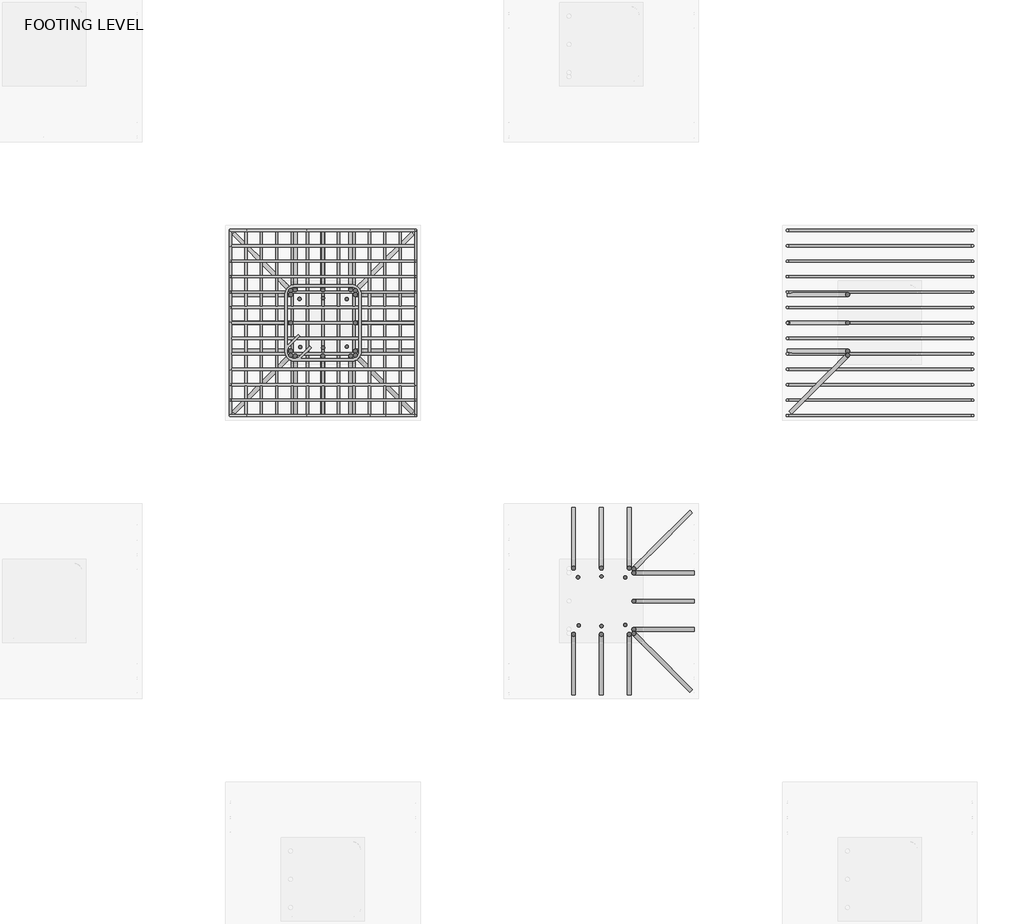
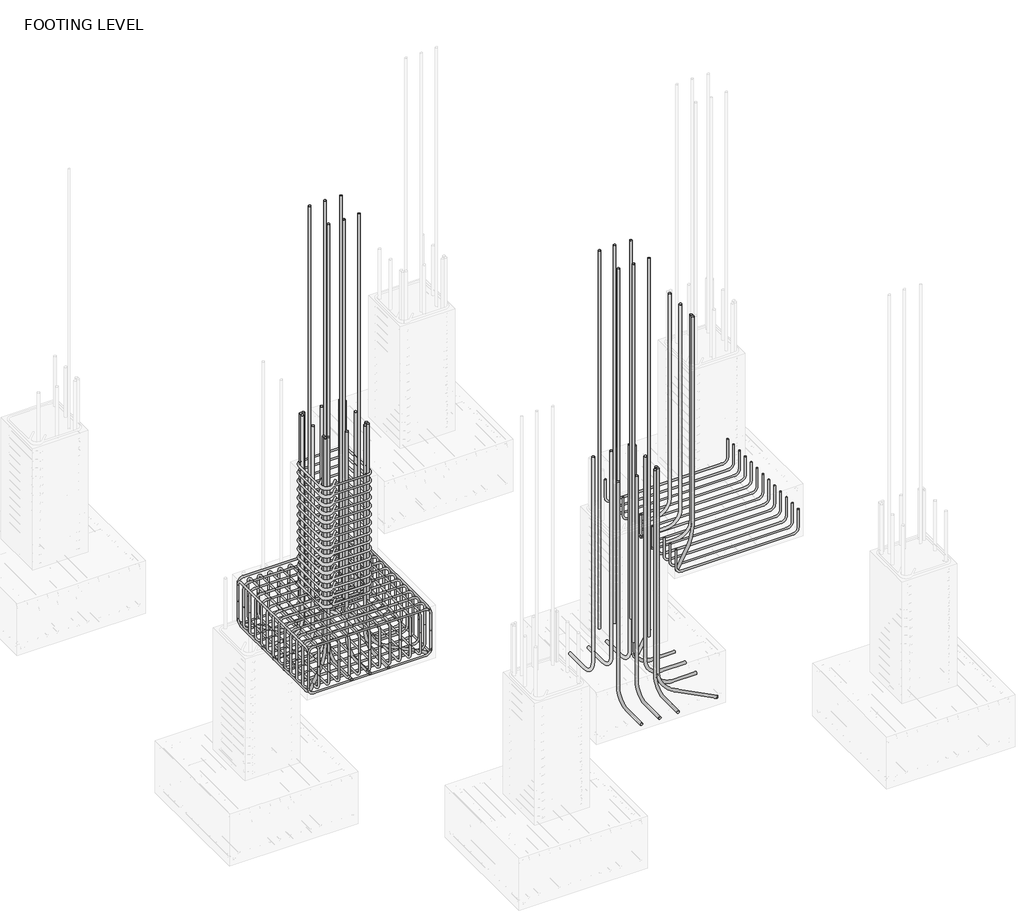
# One storey, part 6 of 10: 34 reinforcing bars.
"""IFC4 building model written with IfcOpenShell, lengths in millimetres."""

from ifc_helpers import new_model, si_unit, point, frame, origin, place, context, project, spatial, polyline, circle_curve, trimmed, segment, composite_curve, source, transform, mapped, element, save
from ifc_brep_helpers import swept_disk

model = new_model("IFC4")

# Units and contexts
model_context = context("Model", 3, world=origin())
ifc_project = project(units=[si_unit("LENGTHUNIT", "METRE", prefix="MILLI")], contexts=[model_context])

# Site, building, storey
site = spatial("IfcSite", under=ifc_project)
building = spatial("IfcBuilding", under=site)
storey = spatial("IfcBuildingStorey", under=building, Name="FOOTING LEVEL", Elevation=-2133.6)

# Reinforcing bars
placement = place(None, origin())
reinforcing_bar_shape = source(origin(), model_context, "Body", "SolidModel", [
    swept_disk(composite_curve([segment(polyline([(365.0730963, 6852.4829396, -2583.0), (365.0730963, 6852.4829396, -2905.1)]), True, "CONTINUOUS"), segment(trimmed(circle_curve(frame((274.8730963, 6852.4829396, -2905.1), z_axis=(0.0, 1.0, 0.0), x_axis=(90.19999999999999, 0.0, 0.0)), 90.2), [point((365.0730963, 6852.4829396, -2905.1))], [point((274.8730963, 6852.4829396, -2995.3))], True, "CARTESIAN"), True, "CONTINUOUS"), segment(polyline([(274.8730963, 6852.4829396, -2995.3), (-1572.9269037, 6852.4829396, -2995.3)]), True, "CONTINUOUS"), segment(trimmed(circle_curve(frame((-1572.9269037, 6852.4829396, -2905.1), z_axis=(0.0, 1.0, 0.0), x_axis=(0.0, 0.0, -90.20000000000027)), 90.2), [point((-1572.9269037, 6852.4829396, -2995.3))], [point((-1663.1269037, 6852.4829396, -2905.1))], True, "CARTESIAN"), True, "CONTINUOUS"), segment(polyline([(-1663.1269037, 6852.4829396, -2905.1), (-1663.1269037, 6852.4829396, -2583.0)]), True, "CONTINUOUS")], self_intersect=False), 12.7),
])
element("IfcReinforcingBar", 1, at=placement, inside=storey, context=model_context, shape_type="MappedRepresentation", body=[
    mapped(reinforcing_bar_shape, transform((0.0, 0.0, 0.0), x_axis=(1.0, 0.0, 0.0), y_axis=(0.0, 1.0, 0.0), z_axis=(0.0, 0.0, 1.0))),
    mapped(reinforcing_bar_shape, transform((0.0, -169.0166667, 0.0), x_axis=(1.0, 0.0, 0.0), y_axis=(0.0, 1.0, 0.0), z_axis=(0.0, 0.0, 1.0))),
    mapped(reinforcing_bar_shape, transform((0.0, -338.0333333, 0.0), x_axis=(1.0, 0.0, 0.0), y_axis=(0.0, 1.0, 0.0), z_axis=(0.0, 0.0, 1.0))),
    mapped(reinforcing_bar_shape, transform((0.0, -507.05, 0.0), x_axis=(1.0, 0.0, 0.0), y_axis=(0.0, 1.0, 0.0), z_axis=(0.0, 0.0, 1.0))),
    mapped(reinforcing_bar_shape, transform((0.0, -676.0666667, 0.0), x_axis=(1.0, 0.0, 0.0), y_axis=(0.0, 1.0, 0.0), z_axis=(0.0, 0.0, 1.0))),
    mapped(reinforcing_bar_shape, transform((0.0, -845.0833333, 0.0), x_axis=(1.0, 0.0, 0.0), y_axis=(0.0, 1.0, 0.0), z_axis=(0.0, 0.0, 1.0))),
    mapped(reinforcing_bar_shape, transform((0.0, -1014.1, 0.0), x_axis=(1.0, 0.0, 0.0), y_axis=(0.0, 1.0, 0.0), z_axis=(0.0, 0.0, 1.0))),
    mapped(reinforcing_bar_shape, transform((0.0, -1183.1166667, 0.0), x_axis=(1.0, 0.0, 0.0), y_axis=(0.0, 1.0, 0.0), z_axis=(0.0, 0.0, 1.0))),
    mapped(reinforcing_bar_shape, transform((0.0, -1352.1333333, 0.0), x_axis=(1.0, 0.0, 0.0), y_axis=(0.0, 1.0, 0.0), z_axis=(0.0, 0.0, 1.0))),
    mapped(reinforcing_bar_shape, transform((0.0, -1521.15, 0.0), x_axis=(1.0, 0.0, 0.0), y_axis=(0.0, 1.0, 0.0), z_axis=(0.0, 0.0, 1.0))),
    mapped(reinforcing_bar_shape, transform((0.0, -1690.1666667, 0.0), x_axis=(1.0, 0.0, 0.0), y_axis=(0.0, 1.0, 0.0), z_axis=(0.0, 0.0, 1.0))),
    mapped(reinforcing_bar_shape, transform((0.0, -1859.1833333, 0.0), x_axis=(1.0, 0.0, 0.0), y_axis=(0.0, 1.0, 0.0), z_axis=(0.0, 0.0, 1.0))),
    mapped(reinforcing_bar_shape, transform((0.0, -2028.2, 0.0), x_axis=(1.0, 0.0, 0.0), y_axis=(0.0, 1.0, 0.0), z_axis=(0.0, 0.0, 1.0))),
])
reinforcing_bar_2_shape = source(origin(), model_context, "Body", "SolidModel", [
    swept_disk(composite_curve([segment(polyline([(-5730.9269037, 6852.4829396, -2583.0), (-5730.9269037, 6852.4829396, -2905.1)]), True, "CONTINUOUS"), segment(trimmed(circle_curve(frame((-5821.1269037, 6852.4829396, -2905.1), z_axis=(0.0, 1.0, 0.0), x_axis=(90.19999999999982, 0.0, 0.0)), 90.2), [point((-5730.9269037, 6852.4829396, -2905.1))], [point((-5821.1269037, 6852.4829396, -2995.3))], True, "CARTESIAN"), True, "CONTINUOUS"), segment(polyline([(-5821.1269037, 6852.4829396, -2995.3), (-7668.9269037, 6852.4829396, -2995.3)]), True, "CONTINUOUS"), segment(trimmed(circle_curve(frame((-7668.9269037, 6852.4829396, -2905.1), z_axis=(0.0, 1.0, 0.0), x_axis=(0.0, 0.0, -90.20000000000027)), 90.2), [point((-7668.9269037, 6852.4829396, -2995.3))], [point((-7759.1269037, 6852.4829396, -2905.1))], True, "CARTESIAN"), True, "CONTINUOUS"), segment(polyline([(-7759.1269037, 6852.4829396, -2905.1), (-7759.1269037, 6852.4829396, -2583.0)]), True, "CONTINUOUS")], self_intersect=False), 12.7),
])
element("IfcReinforcingBar", 2, at=placement, inside=storey, context=model_context, shape_type="MappedRepresentation", body=[
    mapped(reinforcing_bar_2_shape, transform((0.0, 0.0, 0.0), x_axis=(1.0, 0.0, 0.0), y_axis=(0.0, 1.0, 0.0), z_axis=(0.0, 0.0, 1.0))),
    mapped(reinforcing_bar_2_shape, transform((0.0, -169.0166667, 0.0), x_axis=(1.0, 0.0, 0.0), y_axis=(0.0, 1.0, 0.0), z_axis=(0.0, 0.0, 1.0))),
    mapped(reinforcing_bar_2_shape, transform((0.0, -338.0333333, 0.0), x_axis=(1.0, 0.0, 0.0), y_axis=(0.0, 1.0, 0.0), z_axis=(0.0, 0.0, 1.0))),
    mapped(reinforcing_bar_2_shape, transform((0.0, -507.05, 0.0), x_axis=(1.0, 0.0, 0.0), y_axis=(0.0, 1.0, 0.0), z_axis=(0.0, 0.0, 1.0))),
    mapped(reinforcing_bar_2_shape, transform((0.0, -676.0666667, 0.0), x_axis=(1.0, 0.0, 0.0), y_axis=(0.0, 1.0, 0.0), z_axis=(0.0, 0.0, 1.0))),
    mapped(reinforcing_bar_2_shape, transform((0.0, -845.0833333, 0.0), x_axis=(1.0, 0.0, 0.0), y_axis=(0.0, 1.0, 0.0), z_axis=(0.0, 0.0, 1.0))),
    mapped(reinforcing_bar_2_shape, transform((0.0, -1014.1, 0.0), x_axis=(1.0, 0.0, 0.0), y_axis=(0.0, 1.0, 0.0), z_axis=(0.0, 0.0, 1.0))),
    mapped(reinforcing_bar_2_shape, transform((0.0, -1183.1166667, 0.0), x_axis=(1.0, 0.0, 0.0), y_axis=(0.0, 1.0, 0.0), z_axis=(0.0, 0.0, 1.0))),
    mapped(reinforcing_bar_2_shape, transform((0.0, -1352.1333333, 0.0), x_axis=(1.0, 0.0, 0.0), y_axis=(0.0, 1.0, 0.0), z_axis=(0.0, 0.0, 1.0))),
    mapped(reinforcing_bar_2_shape, transform((0.0, -1521.15, 0.0), x_axis=(1.0, 0.0, 0.0), y_axis=(0.0, 1.0, 0.0), z_axis=(0.0, 0.0, 1.0))),
    mapped(reinforcing_bar_2_shape, transform((0.0, -1690.1666667, 0.0), x_axis=(1.0, 0.0, 0.0), y_axis=(0.0, 1.0, 0.0), z_axis=(0.0, 0.0, 1.0))),
    mapped(reinforcing_bar_2_shape, transform((0.0, -1859.1833333, 0.0), x_axis=(1.0, 0.0, 0.0), y_axis=(0.0, 1.0, 0.0), z_axis=(0.0, 0.0, 1.0))),
    mapped(reinforcing_bar_2_shape, transform((0.0, -2028.2, 0.0), x_axis=(1.0, 0.0, 0.0), y_axis=(0.0, 1.0, 0.0), z_axis=(0.0, 0.0, 1.0))),
])
reinforcing_bar_3_shape = source(origin(), model_context, "Body", "SolidModel", [
    swept_disk(composite_curve([segment(polyline([(-7759.1269037, 6852.4829396, -2598.6), (-7759.1269037, 6852.4829396, -2276.5)]), True, "CONTINUOUS"), segment(trimmed(circle_curve(frame((-7668.9269037, 6852.4829396, -2276.5), z_axis=(0.0, 1.0, 0.0), x_axis=(-90.19999999999982, 0.0, 0.0)), 90.2), [point((-7759.1269037, 6852.4829396, -2276.5))], [point((-7668.9269037, 6852.4829396, -2186.3))], True, "CARTESIAN"), True, "CONTINUOUS"), segment(polyline([(-7668.9269037, 6852.4829396, -2186.3), (-5821.1269037, 6852.4829396, -2186.3)]), True, "CONTINUOUS"), segment(trimmed(circle_curve(frame((-5821.1269037, 6852.4829396, -2276.5), z_axis=(0.0, 1.0, 0.0), x_axis=(0.0, 0.0, 90.19999999999982)), 90.2), [point((-5821.1269037, 6852.4829396, -2186.3))], [point((-5730.9269037, 6852.4829396, -2276.5))], True, "CARTESIAN"), True, "CONTINUOUS"), segment(polyline([(-5730.9269037, 6852.4829396, -2276.5), (-5730.9269037, 6852.4829396, -2598.6)]), True, "CONTINUOUS")], self_intersect=False), 12.7),
])
element("IfcReinforcingBar", 3, at=placement, inside=storey, context=model_context, shape_type="MappedRepresentation", body=[
    mapped(reinforcing_bar_3_shape, transform((0.0, 0.0, 0.0), x_axis=(1.0, 0.0, 0.0), y_axis=(0.0, 1.0, 0.0), z_axis=(0.0, 0.0, 1.0))),
    mapped(reinforcing_bar_3_shape, transform((0.0, -169.0166667, 0.0), x_axis=(1.0, 0.0, 0.0), y_axis=(0.0, 1.0, 0.0), z_axis=(0.0, 0.0, 1.0))),
    mapped(reinforcing_bar_3_shape, transform((0.0, -338.0333333, 0.0), x_axis=(1.0, 0.0, 0.0), y_axis=(0.0, 1.0, 0.0), z_axis=(0.0, 0.0, 1.0))),
    mapped(reinforcing_bar_3_shape, transform((0.0, -507.05, 0.0), x_axis=(1.0, 0.0, 0.0), y_axis=(0.0, 1.0, 0.0), z_axis=(0.0, 0.0, 1.0))),
    mapped(reinforcing_bar_3_shape, transform((0.0, -676.0666667, 0.0), x_axis=(1.0, 0.0, 0.0), y_axis=(0.0, 1.0, 0.0), z_axis=(0.0, 0.0, 1.0))),
    mapped(reinforcing_bar_3_shape, transform((0.0, -845.0833333, 0.0), x_axis=(1.0, 0.0, 0.0), y_axis=(0.0, 1.0, 0.0), z_axis=(0.0, 0.0, 1.0))),
    mapped(reinforcing_bar_3_shape, transform((0.0, -1014.1, 0.0), x_axis=(1.0, 0.0, 0.0), y_axis=(0.0, 1.0, 0.0), z_axis=(0.0, 0.0, 1.0))),
    mapped(reinforcing_bar_3_shape, transform((0.0, -1183.1166667, 0.0), x_axis=(1.0, 0.0, 0.0), y_axis=(0.0, 1.0, 0.0), z_axis=(0.0, 0.0, 1.0))),
    mapped(reinforcing_bar_3_shape, transform((0.0, -1352.1333333, 0.0), x_axis=(1.0, 0.0, 0.0), y_axis=(0.0, 1.0, 0.0), z_axis=(0.0, 0.0, 1.0))),
    mapped(reinforcing_bar_3_shape, transform((0.0, -1521.15, 0.0), x_axis=(1.0, 0.0, 0.0), y_axis=(0.0, 1.0, 0.0), z_axis=(0.0, 0.0, 1.0))),
    mapped(reinforcing_bar_3_shape, transform((0.0, -1690.1666667, 0.0), x_axis=(1.0, 0.0, 0.0), y_axis=(0.0, 1.0, 0.0), z_axis=(0.0, 0.0, 1.0))),
    mapped(reinforcing_bar_3_shape, transform((0.0, -1859.1833333, 0.0), x_axis=(1.0, 0.0, 0.0), y_axis=(0.0, 1.0, 0.0), z_axis=(0.0, 0.0, 1.0))),
    mapped(reinforcing_bar_3_shape, transform((0.0, -2028.2, 0.0), x_axis=(1.0, 0.0, 0.0), y_axis=(0.0, 1.0, 0.0), z_axis=(0.0, 0.0, 1.0))),
])
reinforcing_bar_4_shape = source(origin(), model_context, "Body", "SolidModel", [
    swept_disk(composite_curve([segment(polyline([(-5730.9269037, 4824.2829396, -2559.4978077), (-5730.9269037, 4824.2829396, -2881.5978077)]), True, "CONTINUOUS"), segment(trimmed(circle_curve(frame((-5730.9269037, 4914.4829396, -2881.5978077), z_axis=(1.0, 0.0, 0.0), x_axis=(0.0, -90.19999999999982, 0.0)), 90.2), [point((-5730.9269037, 4824.2829396, -2881.5978077))], [point((-5730.9269037, 4914.4829396, -2971.7978077))], True, "CARTESIAN"), True, "CONTINUOUS"), segment(polyline([(-5730.9269037, 4914.4829396, -2971.7978077), (-5730.9269037, 6762.2829396, -2971.7978077)]), True, "CONTINUOUS"), segment(trimmed(circle_curve(frame((-5730.9269037, 6762.2829396, -2881.5978077), z_axis=(1.0, 0.0, 0.0), x_axis=(0.0, 0.0, -90.19999999999982)), 90.2), [point((-5730.9269037, 6762.2829396, -2971.7978077))], [point((-5730.9269037, 6852.4829396, -2881.5978077))], True, "CARTESIAN"), True, "CONTINUOUS"), segment(polyline([(-5730.9269037, 6852.4829396, -2881.5978077), (-5730.9269037, 6852.4829396, -2559.4978077)]), True, "CONTINUOUS")], self_intersect=False), 12.7),
])
element("IfcReinforcingBar", 4, at=placement, inside=storey, context=model_context, shape_type="MappedRepresentation", body=[
    mapped(reinforcing_bar_4_shape, transform((0.0, 0.0, 0.0), x_axis=(1.0, 0.0, 0.0), y_axis=(0.0, 1.0, 0.0), z_axis=(0.0, 0.0, 1.0))),
    mapped(reinforcing_bar_4_shape, transform((-169.0166667, 0.0, 0.0), x_axis=(1.0, 0.0, 0.0), y_axis=(0.0, 1.0, 0.0), z_axis=(0.0, 0.0, 1.0))),
    mapped(reinforcing_bar_4_shape, transform((-338.0333333, 0.0, 0.0), x_axis=(1.0, 0.0, 0.0), y_axis=(0.0, 1.0, 0.0), z_axis=(0.0, 0.0, 1.0))),
    mapped(reinforcing_bar_4_shape, transform((-507.05, 0.0, 0.0), x_axis=(1.0, 0.0, 0.0), y_axis=(0.0, 1.0, 0.0), z_axis=(0.0, 0.0, 1.0))),
    mapped(reinforcing_bar_4_shape, transform((-676.0666667, 0.0, 0.0), x_axis=(1.0, 0.0, 0.0), y_axis=(0.0, 1.0, 0.0), z_axis=(0.0, 0.0, 1.0))),
    mapped(reinforcing_bar_4_shape, transform((-845.0833333, 0.0, 0.0), x_axis=(1.0, 0.0, 0.0), y_axis=(0.0, 1.0, 0.0), z_axis=(0.0, 0.0, 1.0))),
    mapped(reinforcing_bar_4_shape, transform((-1014.1, 0.0, 0.0), x_axis=(1.0, 0.0, 0.0), y_axis=(0.0, 1.0, 0.0), z_axis=(0.0, 0.0, 1.0))),
    mapped(reinforcing_bar_4_shape, transform((-1183.1166667, 0.0, 0.0), x_axis=(1.0, 0.0, 0.0), y_axis=(0.0, 1.0, 0.0), z_axis=(0.0, 0.0, 1.0))),
    mapped(reinforcing_bar_4_shape, transform((-1352.1333333, 0.0, 0.0), x_axis=(1.0, 0.0, 0.0), y_axis=(0.0, 1.0, 0.0), z_axis=(0.0, 0.0, 1.0))),
    mapped(reinforcing_bar_4_shape, transform((-1521.15, 0.0, 0.0), x_axis=(1.0, 0.0, 0.0), y_axis=(0.0, 1.0, 0.0), z_axis=(0.0, 0.0, 1.0))),
    mapped(reinforcing_bar_4_shape, transform((-1690.1666667, 0.0, 0.0), x_axis=(1.0, 0.0, 0.0), y_axis=(0.0, 1.0, 0.0), z_axis=(0.0, 0.0, 1.0))),
    mapped(reinforcing_bar_4_shape, transform((-1859.1833333, 0.0, 0.0), x_axis=(1.0, 0.0, 0.0), y_axis=(0.0, 1.0, 0.0), z_axis=(0.0, 0.0, 1.0))),
    mapped(reinforcing_bar_4_shape, transform((-2028.2, 0.0, 0.0), x_axis=(1.0, 0.0, 0.0), y_axis=(0.0, 1.0, 0.0), z_axis=(0.0, 0.0, 1.0))),
])
reinforcing_bar_5_shape = source(origin(), model_context, "Body", "SolidModel", [
    swept_disk(composite_curve([segment(polyline([(-7759.1269037, 4824.2829396, -2622.9919875), (-7759.1269037, 4824.2829396, -2300.8919875)]), True, "CONTINUOUS"), segment(trimmed(circle_curve(frame((-7759.1269037, 4914.4829396, -2300.8919875), z_axis=(-1.0, 0.0, 0.0), x_axis=(0.0, -90.19999999999982, 0.0)), 90.2), [point((-7759.1269037, 4824.2829396, -2300.8919875))], [point((-7759.1269037, 4914.4829396, -2210.6919875))], True, "CARTESIAN"), True, "CONTINUOUS"), segment(polyline([(-7759.1269037, 4914.4829396, -2210.6919875), (-7759.1269037, 6762.2829396, -2210.6919875)]), True, "CONTINUOUS"), segment(trimmed(circle_curve(frame((-7759.1269037, 6762.2829396, -2300.8919875), z_axis=(-1.0, 0.0, 0.0), x_axis=(0.0, 0.0, 90.20000000000027)), 90.2), [point((-7759.1269037, 6762.2829396, -2210.6919875))], [point((-7759.1269037, 6852.4829396, -2300.8919875))], True, "CARTESIAN"), True, "CONTINUOUS"), segment(polyline([(-7759.1269037, 6852.4829396, -2300.8919875), (-7759.1269037, 6852.4829396, -2622.9919875)]), True, "CONTINUOUS")], self_intersect=False), 12.7),
])
element("IfcReinforcingBar", 5, at=placement, inside=storey, context=model_context, shape_type="MappedRepresentation", body=[
    mapped(reinforcing_bar_5_shape, transform((0.0, 0.0, 0.0), x_axis=(1.0, 0.0, 0.0), y_axis=(0.0, 1.0, 0.0), z_axis=(0.0, 0.0, 1.0))),
    mapped(reinforcing_bar_5_shape, transform((169.0166667, 0.0, 0.0), x_axis=(1.0, 0.0, 0.0), y_axis=(0.0, 1.0, 0.0), z_axis=(0.0, 0.0, 1.0))),
    mapped(reinforcing_bar_5_shape, transform((338.0333333, 0.0, 0.0), x_axis=(1.0, 0.0, 0.0), y_axis=(0.0, 1.0, 0.0), z_axis=(0.0, 0.0, 1.0))),
    mapped(reinforcing_bar_5_shape, transform((507.05, 0.0, 0.0), x_axis=(1.0, 0.0, 0.0), y_axis=(0.0, 1.0, 0.0), z_axis=(0.0, 0.0, 1.0))),
    mapped(reinforcing_bar_5_shape, transform((676.0666667, 0.0, 0.0), x_axis=(1.0, 0.0, 0.0), y_axis=(0.0, 1.0, 0.0), z_axis=(0.0, 0.0, 1.0))),
    mapped(reinforcing_bar_5_shape, transform((845.0833333, 0.0, 0.0), x_axis=(1.0, 0.0, 0.0), y_axis=(0.0, 1.0, 0.0), z_axis=(0.0, 0.0, 1.0))),
    mapped(reinforcing_bar_5_shape, transform((1014.1, 0.0, 0.0), x_axis=(1.0, 0.0, 0.0), y_axis=(0.0, 1.0, 0.0), z_axis=(0.0, 0.0, 1.0))),
    mapped(reinforcing_bar_5_shape, transform((1183.1166667, 0.0, 0.0), x_axis=(1.0, 0.0, 0.0), y_axis=(0.0, 1.0, 0.0), z_axis=(0.0, 0.0, 1.0))),
    mapped(reinforcing_bar_5_shape, transform((1352.1333333, 0.0, 0.0), x_axis=(1.0, 0.0, 0.0), y_axis=(0.0, 1.0, 0.0), z_axis=(0.0, 0.0, 1.0))),
    mapped(reinforcing_bar_5_shape, transform((1521.15, 0.0, 0.0), x_axis=(1.0, 0.0, 0.0), y_axis=(0.0, 1.0, 0.0), z_axis=(0.0, 0.0, 1.0))),
    mapped(reinforcing_bar_5_shape, transform((1690.1666667, 0.0, 0.0), x_axis=(1.0, 0.0, 0.0), y_axis=(0.0, 1.0, 0.0), z_axis=(0.0, 0.0, 1.0))),
    mapped(reinforcing_bar_5_shape, transform((1859.1833333, 0.0, 0.0), x_axis=(1.0, 0.0, 0.0), y_axis=(0.0, 1.0, 0.0), z_axis=(0.0, 0.0, 1.0))),
    mapped(reinforcing_bar_5_shape, transform((2028.2, 0.0, 0.0), x_axis=(1.0, 0.0, 0.0), y_axis=(0.0, 1.0, 0.0), z_axis=(0.0, 0.0, 1.0))),
])
reinforcing_bar_6_shape = source(origin(), model_context, "Body", "SolidModel", [
    swept_disk(composite_curve([segment(polyline([(-6882.1462687, 5573.7015113, 0.0), (-6995.545872, 5460.3019079, 0.0)]), True, "CONTINUOUS"), segment(trimmed(circle_curve(frame((-7059.3269037, 5524.0829396, 0.0), z_axis=(0.0, 0.0, -1.0), x_axis=(63.78103170000031, -63.78103170000031, 0.0)), 90.2), [point((-6995.545872, 5460.3019079, 0.0))], [point((-7149.5269037, 5524.0829396, 0.0))], True, "CARTESIAN"), True, "CONTINUOUS"), segment(polyline([(-7149.5269037, 5524.0829396, 0.0), (-7149.5269037, 6152.6829396, 0.0)]), True, "CONTINUOUS"), segment(trimmed(circle_curve(frame((-7059.3269037, 6152.6829396, 0.0), z_axis=(0.0, 0.0, -1.0), x_axis=(-90.19999999999982, 0.0, 0.0)), 90.2), [point((-7149.5269037, 6152.6829396, 0.0))], [point((-7059.3269037, 6242.8829396, 0.0))], True, "CARTESIAN"), True, "CONTINUOUS"), segment(polyline([(-7059.3269037, 6242.8829396, 0.0), (-6430.7269037, 6242.8829396, 0.0)]), True, "CONTINUOUS"), segment(trimmed(circle_curve(frame((-6430.7269037, 6152.7273645, 2.8305953), z_axis=(0.0, -0.03138132276777647, -0.9995074850051623), x_axis=(0.0, 90.15557510000053, -2.8305953)), 90.2), [point((-6430.7269037, 6242.8829396, 0.0))], [point((-6340.5269037, 6152.7273645, 2.8305953))], True, "CARTESIAN"), True, "CONTINUOUS"), segment(polyline([(-6340.5269037, 6152.7273645, 2.8305953), (-6340.5269037, 5524.0385147, 22.5694047)]), True, "CONTINUOUS"), segment(trimmed(circle_curve(frame((-6430.7269037, 5524.0385147, 22.5694047), z_axis=(0.0, -0.03138132276777647, -0.9995074850051623), x_axis=(90.19999999999982, 0.0, 0.0)), 90.2), [point((-6340.5269037, 5524.0385147, 22.5694047))], [point((-6430.7269037, 5433.8829396, 25.4))], True, "CARTESIAN"), True, "CONTINUOUS"), segment(polyline([(-6430.7269037, 5433.8829396, 25.4), (-7059.3269037, 5433.8829396, 25.4)]), True, "CONTINUOUS"), segment(trimmed(circle_curve(frame((-7059.3269037, 5524.0829396, 25.4), z_axis=(0.0, 0.0, -1.0), x_axis=(0.0, -90.19999999999982, 0.0)), 90.2), [point((-7059.3269037, 5433.8829396, 25.4))], [point((-7123.1079353, 5587.8639713, 25.4))], True, "CARTESIAN"), True, "CONTINUOUS"), segment(polyline([(-7123.1079353, 5587.8639713, 25.4), (-7009.708332, 5701.2635746, 25.4)]), True, "CONTINUOUS")], self_intersect=False), 12.7),
])
element("IfcReinforcingBar", 6, at=placement, inside=storey, context=model_context, shape_type="MappedRepresentation", body=[
    mapped(reinforcing_bar_6_shape, transform((0.0, 0.0, 0.0), x_axis=(1.0, 0.0, 0.0), y_axis=(0.0, 1.0, 0.0), z_axis=(0.0, 0.0, 1.0))),
    mapped(reinforcing_bar_6_shape, transform((0.0, 0.0, -148.6357143), x_axis=(1.0, 0.0, 0.0), y_axis=(0.0, 1.0, 0.0), z_axis=(0.0, 0.0, 1.0))),
    mapped(reinforcing_bar_6_shape, transform((0.0, 0.0, -297.2714286), x_axis=(1.0, 0.0, 0.0), y_axis=(0.0, 1.0, 0.0), z_axis=(0.0, 0.0, 1.0))),
    mapped(reinforcing_bar_6_shape, transform((0.0, 0.0, -445.9071429), x_axis=(1.0, 0.0, 0.0), y_axis=(0.0, 1.0, 0.0), z_axis=(0.0, 0.0, 1.0))),
    mapped(reinforcing_bar_6_shape, transform((0.0, 0.0, -594.5428571), x_axis=(1.0, 0.0, 0.0), y_axis=(0.0, 1.0, 0.0), z_axis=(0.0, 0.0, 1.0))),
    mapped(reinforcing_bar_6_shape, transform((0.0, 0.0, -743.1785714), x_axis=(1.0, 0.0, 0.0), y_axis=(0.0, 1.0, 0.0), z_axis=(0.0, 0.0, 1.0))),
    mapped(reinforcing_bar_6_shape, transform((0.0, 0.0, -891.8142857), x_axis=(1.0, 0.0, 0.0), y_axis=(0.0, 1.0, 0.0), z_axis=(0.0, 0.0, 1.0))),
    mapped(reinforcing_bar_6_shape, transform((0.0, 0.0, -1040.45), x_axis=(1.0, 0.0, 0.0), y_axis=(0.0, 1.0, 0.0), z_axis=(0.0, 0.0, 1.0))),
    mapped(reinforcing_bar_6_shape, transform((0.0, 0.0, -1189.0857143), x_axis=(1.0, 0.0, 0.0), y_axis=(0.0, 1.0, 0.0), z_axis=(0.0, 0.0, 1.0))),
    mapped(reinforcing_bar_6_shape, transform((0.0, 0.0, -1337.7214286), x_axis=(1.0, 0.0, 0.0), y_axis=(0.0, 1.0, 0.0), z_axis=(0.0, 0.0, 1.0))),
    mapped(reinforcing_bar_6_shape, transform((0.0, 0.0, -1486.3571429), x_axis=(1.0, 0.0, 0.0), y_axis=(0.0, 1.0, 0.0), z_axis=(0.0, 0.0, 1.0))),
    mapped(reinforcing_bar_6_shape, transform((0.0, 0.0, -1634.9928571), x_axis=(1.0, 0.0, 0.0), y_axis=(0.0, 1.0, 0.0), z_axis=(0.0, 0.0, 1.0))),
    mapped(reinforcing_bar_6_shape, transform((0.0, 0.0, -1783.6285714), x_axis=(1.0, 0.0, 0.0), y_axis=(0.0, 1.0, 0.0), z_axis=(0.0, 0.0, 1.0))),
    mapped(reinforcing_bar_6_shape, transform((0.0, 0.0, -1932.2642857), x_axis=(1.0, 0.0, 0.0), y_axis=(0.0, 1.0, 0.0), z_axis=(0.0, 0.0, 1.0))),
    mapped(reinforcing_bar_6_shape, transform((0.0, 0.0, -2080.9), x_axis=(1.0, 0.0, 0.0), y_axis=(0.0, 1.0, 0.0), z_axis=(0.0, 0.0, 1.0))),
])
element("IfcReinforcingBar", 7, at=placement, inside=storey, context=model_context, shape_type="SolidModel", body=[
    swept_disk(composite_curve([segment(polyline([(-1629.4807966, 4857.9290467, -2976.5), (-1182.5300058, 5304.8798374, -2976.5)]), True, "CONTINUOUS"), segment(trimmed(circle_curve(frame((-1182.5300058, 5304.8798374, -2722.5), z_axis=(0.7071067811865475, -0.7071067811865477, 0.0), x_axis=(0.0, 0.0, -254.0)), 254.0), [point((-1182.5300058, 5304.8798374, -2976.5))], [point((-1002.9248834, 5484.4849599, -2722.5))], True, "CARTESIAN"), True, "CONTINUOUS"), segment(polyline([(-1002.9248834, 5484.4849599, -2722.5), (-1002.9248834, 5484.4849599, 874.4)]), True, "CONTINUOUS")], self_intersect=False), 21.5),
])
reinforcing_bar_7_shape = source(origin(), model_context, "Body", "SolidModel", [
    swept_disk(composite_curve([segment(polyline([(-1665.8269037, 5530.0019966, -2976.5), (-1256.9248834, 5530.0019966, -2976.5)]), True, "CONTINUOUS"), segment(trimmed(circle_curve(frame((-1256.9248834, 5530.0019966, -2722.5), z_axis=(0.0, -1.0, 0.0), x_axis=(0.0, 0.0, -254.0)), 254.0), [point((-1256.9248834, 5530.0019966, -2976.5))], [point((-1002.9248834, 5530.0019966, -2722.5))], True, "CARTESIAN"), True, "CONTINUOUS"), segment(polyline([(-1002.9248834, 5530.0019966, -2722.5), (-1002.9248834, 5530.0019966, 874.4)]), True, "CONTINUOUS")], self_intersect=False), 21.5),
])
element("IfcReinforcingBar", 8, at=placement, inside=storey, context=model_context, shape_type="MappedRepresentation", body=[
    mapped(reinforcing_bar_7_shape, transform((0.0, 0.0, 0.0), x_axis=(1.0, 0.0, 0.0), y_axis=(0.0, 1.0, 0.0), z_axis=(0.0, 0.0, 1.0))),
    mapped(reinforcing_bar_7_shape, transform((0.0, 309.128507, 0.0), x_axis=(1.0, 0.0, 0.0), y_axis=(0.0, 1.0, 0.0), z_axis=(0.0, 0.0, 1.0))),
    mapped(reinforcing_bar_7_shape, transform((0.0, 618.2570139, 0.0), x_axis=(1.0, 0.0, 0.0), y_axis=(0.0, 1.0, 0.0), z_axis=(0.0, 0.0, 1.0))),
])
element("IfcReinforcingBar", 9, at=placement, inside=storey, context=model_context, shape_type="SolidModel", body=[
    swept_disk(composite_curve([segment(polyline([(-2716.5730107, 3770.8368325, -2976.5), (-3163.5238015, 3323.8860418, -2976.5)]), True, "CONTINUOUS"), segment(trimmed(circle_curve(frame((-3163.5238015, 3323.8860418, -2722.5), z_axis=(-0.7071067811865475, 0.7071067811865477, 0.0), x_axis=(0.0, 0.0, -254.0)), 254.0), [point((-3163.5238015, 3323.8860418, -2976.5))], [point((-3343.1289239, 3144.2809193, -2722.5))], True, "CARTESIAN"), True, "CONTINUOUS"), segment(polyline([(-3343.1289239, 3144.2809193, -2722.5), (-3343.1289239, 3144.2809193, 874.4)]), True, "CONTINUOUS")], self_intersect=False), 21.5),
])
element("IfcReinforcingBar", 10, at=placement, inside=storey, context=model_context, shape_type="SolidModel", body=[
    swept_disk(composite_curve([segment(polyline([(-2716.5730107, 1809.9290467, -2976.5), (-3163.5238015, 2256.8798374, -2976.5)]), True, "CONTINUOUS"), segment(trimmed(circle_curve(frame((-3163.5238015, 2256.8798374, -2722.5), z_axis=(0.7071067811865508, 0.7071067811865444, 0.0), x_axis=(0.0, 0.0, -254.0)), 254.0), [point((-3163.5238015, 2256.8798374, -2976.5))], [point((-3343.1289239, 2436.4849599, -2722.5))], True, "CARTESIAN"), True, "CONTINUOUS"), segment(polyline([(-3343.1289239, 2436.4849599, -2722.5), (-3343.1289239, 2436.4849599, 874.4)]), True, "CONTINUOUS")], self_intersect=False), 21.5),
])
reinforcing_bar_8_shape = source(origin(), model_context, "Body", "SolidModel", [
    swept_disk(composite_curve([segment(polyline([(-2680.2269037, 2482.0019966, -2976.5), (-3089.1289239, 2482.0019966, -2976.5)]), True, "CONTINUOUS"), segment(trimmed(circle_curve(frame((-3089.1289239, 2482.0019966, -2722.5), z_axis=(0.0, 1.0, 0.0), x_axis=(0.0, 0.0, -254.0)), 254.0), [point((-3089.1289239, 2482.0019966, -2976.5))], [point((-3343.1289239, 2482.0019966, -2722.5))], True, "CARTESIAN"), True, "CONTINUOUS"), segment(polyline([(-3343.1289239, 2482.0019966, -2722.5), (-3343.1289239, 2482.0019966, 874.4)]), True, "CONTINUOUS")], self_intersect=False), 21.5),
])
element("IfcReinforcingBar", 11, at=placement, inside=storey, context=model_context, shape_type="MappedRepresentation", body=[
    mapped(reinforcing_bar_8_shape, transform((0.0, 0.0, 0.0), x_axis=(1.0, 0.0, 0.0), y_axis=(0.0, 1.0, 0.0), z_axis=(0.0, 0.0, 1.0))),
    mapped(reinforcing_bar_8_shape, transform((0.0, 309.128507, 0.0), x_axis=(1.0, 0.0, 0.0), y_axis=(0.0, 1.0, 0.0), z_axis=(0.0, 0.0, 1.0))),
    mapped(reinforcing_bar_8_shape, transform((0.0, 618.2570139, 0.0), x_axis=(1.0, 0.0, 0.0), y_axis=(0.0, 1.0, 0.0), z_axis=(0.0, 0.0, 1.0))),
])
reinforcing_bar_9_shape = source(origin(), model_context, "Body", "SolidModel", [
    swept_disk(composite_curve([segment(polyline([(-3393.6587573, 3815.4257505, -2976.5), (-3393.6587573, 3406.5237302, -2976.5)]), True, "CONTINUOUS"), segment(trimmed(circle_curve(frame((-3393.6587573, 3406.5237302, -2722.5), z_axis=(-1.0, 0.0, 0.0), x_axis=(0.0, 0.0, -254.0)), 254.0), [point((-3393.6587573, 3406.5237302, -2976.5))], [point((-3393.6587573, 3152.5237302, -2722.5))], True, "CARTESIAN"), True, "CONTINUOUS"), segment(polyline([(-3393.6587573, 3152.5237302, -2722.5), (-3393.6587573, 3152.5237302, 874.4)]), True, "CONTINUOUS")], self_intersect=False), 21.5),
])
element("IfcReinforcingBar", 12, at=placement, inside=storey, context=model_context, shape_type="MappedRepresentation", body=[
    mapped(reinforcing_bar_9_shape, transform((0.0, 0.0, 0.0), x_axis=(1.0, 0.0, 0.0), y_axis=(0.0, 1.0, 0.0), z_axis=(0.0, 0.0, 1.0))),
    mapped(reinforcing_bar_9_shape, transform((-304.9765997, 0.0, 0.0), x_axis=(1.0, 0.0, 0.0), y_axis=(0.0, 1.0, 0.0), z_axis=(0.0, 0.0, 1.0))),
    mapped(reinforcing_bar_9_shape, transform((-609.9531995, 0.0, 0.0), x_axis=(1.0, 0.0, 0.0), y_axis=(0.0, 1.0, 0.0), z_axis=(0.0, 0.0, 1.0))),
])
reinforcing_bar_10_shape = source(origin(), model_context, "Body", "SolidModel", [
    swept_disk(composite_curve([segment(polyline([(-3393.6587573, 1765.3401287, -2976.5), (-3393.6587573, 2174.242149, -2976.5)]), True, "CONTINUOUS"), segment(trimmed(circle_curve(frame((-3393.6587573, 2174.242149, -2722.5), z_axis=(1.0, 0.0, 0.0), x_axis=(0.0, 0.0, -254.0)), 254.0), [point((-3393.6587573, 2174.242149, -2976.5))], [point((-3393.6587573, 2428.242149, -2722.5))], True, "CARTESIAN"), True, "CONTINUOUS"), segment(polyline([(-3393.6587573, 2428.242149, -2722.5), (-3393.6587573, 2428.242149, 874.4)]), True, "CONTINUOUS")], self_intersect=False), 21.5),
])
element("IfcReinforcingBar", 13, at=placement, inside=storey, context=model_context, shape_type="MappedRepresentation", body=[
    mapped(reinforcing_bar_10_shape, transform((0.0, 0.0, 0.0), x_axis=(1.0, 0.0, 0.0), y_axis=(0.0, 1.0, 0.0), z_axis=(0.0, 0.0, 1.0))),
    mapped(reinforcing_bar_10_shape, transform((-304.9765997, 0.0, 0.0), x_axis=(1.0, 0.0, 0.0), y_axis=(0.0, 1.0, 0.0), z_axis=(0.0, 0.0, 1.0))),
    mapped(reinforcing_bar_10_shape, transform((-609.9531995, 0.0, 0.0), x_axis=(1.0, 0.0, 0.0), y_axis=(0.0, 1.0, 0.0), z_axis=(0.0, 0.0, 1.0))),
])
element("IfcReinforcingBar", 14, at=placement, inside=storey, context=model_context, shape_type="SolidModel", body=[
    swept_disk(composite_curve([segment(polyline([(-5764.5730107, 4857.9290467, -2976.5), (-6211.5238015, 5304.8798374, -2976.5)]), True, "CONTINUOUS"), segment(trimmed(circle_curve(frame((-6211.5238015, 5304.8798374, -2722.5), z_axis=(0.7071067811865508, 0.7071067811865444, 0.0), x_axis=(0.0, 0.0, -254.0)), 254.0), [point((-6211.5238015, 5304.8798374, -2976.5))], [point((-6391.1289239, 5484.4849599, -2722.5))], True, "CARTESIAN"), True, "CONTINUOUS"), segment(polyline([(-6391.1289239, 5484.4849599, -2722.5), (-6391.1289239, 5484.4849599, 874.4)]), True, "CONTINUOUS")], self_intersect=False), 21.5),
])
element("IfcReinforcingBar", 15, at=placement, inside=storey, context=model_context, shape_type="SolidModel", body=[
    swept_disk(composite_curve([segment(polyline([(-7725.4807966, 4857.9290467, -2976.5), (-7278.5300058, 5304.8798374, -2976.5)]), True, "CONTINUOUS"), segment(trimmed(circle_curve(frame((-7278.5300058, 5304.8798374, -2722.5), z_axis=(0.7071067811865475, -0.7071067811865477, 0.0), x_axis=(0.0, 0.0, -254.0)), 254.0), [point((-7278.5300058, 5304.8798374, -2976.5))], [point((-7098.9248834, 5484.4849599, -2722.5))], True, "CARTESIAN"), True, "CONTINUOUS"), segment(polyline([(-7098.9248834, 5484.4849599, -2722.5), (-7098.9248834, 5484.4849599, 874.4)]), True, "CONTINUOUS")], self_intersect=False), 21.5),
])
element("IfcReinforcingBar", 16, at=placement, inside=storey, context=model_context, shape_type="SolidModel", body=[
    swept_disk(composite_curve([segment(polyline([(-5764.5730107, 6818.8368325, -2976.5), (-6211.5238015, 6371.8860418, -2976.5)]), True, "CONTINUOUS"), segment(trimmed(circle_curve(frame((-6211.5238015, 6371.8860418, -2722.5), z_axis=(-0.7071067811865475, 0.7071067811865477, 0.0), x_axis=(0.0, 0.0, -254.0)), 254.0), [point((-6211.5238015, 6371.8860418, -2976.5))], [point((-6391.1289239, 6192.2809193, -2722.5))], True, "CARTESIAN"), True, "CONTINUOUS"), segment(polyline([(-6391.1289239, 6192.2809193, -2722.5), (-6391.1289239, 6192.2809193, 874.4)]), True, "CONTINUOUS")], self_intersect=False), 21.5),
])
element("IfcReinforcingBar", 17, at=placement, inside=storey, context=model_context, shape_type="SolidModel", body=[
    swept_disk(composite_curve([segment(polyline([(-7725.4807966, 6818.8368325, -2976.5), (-7278.5300058, 6371.8860418, -2976.5)]), True, "CONTINUOUS"), segment(trimmed(circle_curve(frame((-7278.5300058, 6371.8860418, -2722.5), z_axis=(-0.7071067811865508, -0.7071067811865444, 0.0), x_axis=(0.0, 0.0, -254.0)), 254.0), [point((-7278.5300058, 6371.8860418, -2976.5))], [point((-7098.9248834, 6192.2809193, -2722.5))], True, "CARTESIAN"), True, "CONTINUOUS"), segment(polyline([(-7098.9248834, 6192.2809193, -2722.5), (-7098.9248834, 6192.2809193, 874.4)]), True, "CONTINUOUS")], self_intersect=False), 21.5),
])
element("IfcReinforcingBar", 18, at=placement, inside=storey, context=model_context, shape_type="SolidModel", body=[
    swept_disk(composite_curve([segment(polyline([(-5764.5730107, 4857.9290467, -2976.5), (-6211.5238015, 5304.8798374, -2976.5)]), True, "CONTINUOUS"), segment(trimmed(circle_curve(frame((-6211.5238015, 5304.8798374, -2722.5), z_axis=(0.7071067811865508, 0.7071067811865444, 0.0), x_axis=(0.0, 0.0, -254.0)), 254.0), [point((-6211.5238015, 5304.8798374, -2976.5))], [point((-6391.1289239, 5484.4849599, -2722.5))], True, "CARTESIAN"), True, "CONTINUOUS"), segment(polyline([(-6391.1289239, 5484.4849599, -2722.5), (-6391.1289239, 5484.4849599, 874.4)]), True, "CONTINUOUS")], self_intersect=False), 21.5),
])
reinforcing_bar_11_shape = source(origin(), model_context, "Body", "SolidModel", [
    swept_disk(composite_curve([segment(polyline([(-5728.2269037, 5530.0019966, -2976.5), (-6137.1289239, 5530.0019966, -2976.5)]), True, "CONTINUOUS"), segment(trimmed(circle_curve(frame((-6137.1289239, 5530.0019966, -2722.5), z_axis=(0.0, 1.0, 0.0), x_axis=(0.0, 0.0, -254.0)), 254.0), [point((-6137.1289239, 5530.0019966, -2976.5))], [point((-6391.1289239, 5530.0019966, -2722.5))], True, "CARTESIAN"), True, "CONTINUOUS"), segment(polyline([(-6391.1289239, 5530.0019966, -2722.5), (-6391.1289239, 5530.0019966, 874.4)]), True, "CONTINUOUS")], self_intersect=False), 21.5),
])
element("IfcReinforcingBar", 19, at=placement, inside=storey, context=model_context, shape_type="MappedRepresentation", body=[
    mapped(reinforcing_bar_11_shape, transform((0.0, 0.0, 0.0), x_axis=(1.0, 0.0, 0.0), y_axis=(0.0, 1.0, 0.0), z_axis=(0.0, 0.0, 1.0))),
    mapped(reinforcing_bar_11_shape, transform((0.0, 309.128507, 0.0), x_axis=(1.0, 0.0, 0.0), y_axis=(0.0, 1.0, 0.0), z_axis=(0.0, 0.0, 1.0))),
    mapped(reinforcing_bar_11_shape, transform((0.0, 618.2570139, 0.0), x_axis=(1.0, 0.0, 0.0), y_axis=(0.0, 1.0, 0.0), z_axis=(0.0, 0.0, 1.0))),
])
reinforcing_bar_12_shape = source(origin(), model_context, "Body", "SolidModel", [
    swept_disk(composite_curve([segment(polyline([(-7761.8269037, 5530.0019966, -2976.5), (-7352.9248834, 5530.0019966, -2976.5)]), True, "CONTINUOUS"), segment(trimmed(circle_curve(frame((-7352.9248834, 5530.0019966, -2722.5), z_axis=(0.0, -1.0, 0.0), x_axis=(0.0, 0.0, -254.0)), 254.0), [point((-7352.9248834, 5530.0019966, -2976.5))], [point((-7098.9248834, 5530.0019966, -2722.5))], True, "CARTESIAN"), True, "CONTINUOUS"), segment(polyline([(-7098.9248834, 5530.0019966, -2722.5), (-7098.9248834, 5530.0019966, 874.4)]), True, "CONTINUOUS")], self_intersect=False), 21.5),
])
element("IfcReinforcingBar", 20, at=placement, inside=storey, context=model_context, shape_type="MappedRepresentation", body=[
    mapped(reinforcing_bar_12_shape, transform((0.0, 0.0, 0.0), x_axis=(1.0, 0.0, 0.0), y_axis=(0.0, 1.0, 0.0), z_axis=(0.0, 0.0, 1.0))),
    mapped(reinforcing_bar_12_shape, transform((0.0, 309.128507, 0.0), x_axis=(1.0, 0.0, 0.0), y_axis=(0.0, 1.0, 0.0), z_axis=(0.0, 0.0, 1.0))),
    mapped(reinforcing_bar_12_shape, transform((0.0, 618.2570139, 0.0), x_axis=(1.0, 0.0, 0.0), y_axis=(0.0, 1.0, 0.0), z_axis=(0.0, 0.0, 1.0))),
])
reinforcing_bar_13_shape = source(origin(), model_context, "Body", "SolidModel", [
    swept_disk(composite_curve([segment(polyline([(-6441.6587573, 6863.4257505, -2976.5), (-6441.6587573, 6454.5237302, -2976.5)]), True, "CONTINUOUS"), segment(trimmed(circle_curve(frame((-6441.6587573, 6454.5237302, -2722.5), z_axis=(-1.0, 0.0, 0.0), x_axis=(0.0, 0.0, -254.0)), 254.0), [point((-6441.6587573, 6454.5237302, -2976.5))], [point((-6441.6587573, 6200.5237302, -2722.5))], True, "CARTESIAN"), True, "CONTINUOUS"), segment(polyline([(-6441.6587573, 6200.5237302, -2722.5), (-6441.6587573, 6200.5237302, 874.4)]), True, "CONTINUOUS")], self_intersect=False), 21.5),
])
element("IfcReinforcingBar", 21, at=placement, inside=storey, context=model_context, shape_type="MappedRepresentation", body=[
    mapped(reinforcing_bar_13_shape, transform((0.0, 0.0, 0.0), x_axis=(1.0, 0.0, 0.0), y_axis=(0.0, 1.0, 0.0), z_axis=(0.0, 0.0, 1.0))),
    mapped(reinforcing_bar_13_shape, transform((-304.9765997, 0.0, 0.0), x_axis=(1.0, 0.0, 0.0), y_axis=(0.0, 1.0, 0.0), z_axis=(0.0, 0.0, 1.0))),
    mapped(reinforcing_bar_13_shape, transform((-609.9531995, 0.0, 0.0), x_axis=(1.0, 0.0, 0.0), y_axis=(0.0, 1.0, 0.0), z_axis=(0.0, 0.0, 1.0))),
])
reinforcing_bar_14_shape = source(origin(), model_context, "Body", "SolidModel", [
    swept_disk(composite_curve([segment(polyline([(-6441.6587573, 4813.3401287, -2976.5), (-6441.6587573, 5222.242149, -2976.5)]), True, "CONTINUOUS"), segment(trimmed(circle_curve(frame((-6441.6587573, 5222.242149, -2722.5), z_axis=(1.0, 0.0, 0.0), x_axis=(0.0, 0.0, -254.0)), 254.0), [point((-6441.6587573, 5222.242149, -2976.5))], [point((-6441.6587573, 5476.242149, -2722.5))], True, "CARTESIAN"), True, "CONTINUOUS"), segment(polyline([(-6441.6587573, 5476.242149, -2722.5), (-6441.6587573, 5476.242149, 874.4)]), True, "CONTINUOUS")], self_intersect=False), 21.5),
])
element("IfcReinforcingBar", 22, at=placement, inside=storey, context=model_context, shape_type="MappedRepresentation", body=[
    mapped(reinforcing_bar_14_shape, transform((0.0, 0.0, 0.0), x_axis=(1.0, 0.0, 0.0), y_axis=(0.0, 1.0, 0.0), z_axis=(0.0, 0.0, 1.0))),
    mapped(reinforcing_bar_14_shape, transform((-304.9765997, 0.0, 0.0), x_axis=(1.0, 0.0, 0.0), y_axis=(0.0, 1.0, 0.0), z_axis=(0.0, 0.0, 1.0))),
    mapped(reinforcing_bar_14_shape, transform((-609.9531995, 0.0, 0.0), x_axis=(1.0, 0.0, 0.0), y_axis=(0.0, 1.0, 0.0), z_axis=(0.0, 0.0, 1.0))),
])
element("IfcReinforcingBar", 23, at=placement, inside=storey, context=model_context, shape_type="SolidModel", body=[
    swept_disk(composite_curve([segment(polyline([(-6485.0269037, 6098.3829396, 4538.8488542), (-6485.0269037, 6098.3829396, -2093.6)]), True, "CONTINUOUS")], self_intersect=False), 17.9),
])
element("IfcReinforcingBar", 24, at=placement, inside=storey, context=model_context, shape_type="SolidModel", body=[
    swept_disk(composite_curve([segment(polyline([(-7002.5269037, 6100.8829396, 4538.8488542), (-7002.5269037, 6100.8829396, -2093.6)]), True, "CONTINUOUS")], self_intersect=False), 17.9),
])
element("IfcReinforcingBar", 25, at=placement, inside=storey, context=model_context, shape_type="SolidModel", body=[
    swept_disk(composite_curve([segment(polyline([(-6485.0269037, 5578.3829396, 4538.8488542), (-6485.0269037, 5578.3829396, -2093.6)]), True, "CONTINUOUS")], self_intersect=False), 17.9),
])
element("IfcReinforcingBar", 26, at=placement, inside=storey, context=model_context, shape_type="SolidModel", body=[
    swept_disk(composite_curve([segment(polyline([(-6995.0269037, 5573.3829396, 4538.8488542), (-6995.0269037, 5573.3829396, -2093.6)]), True, "CONTINUOUS")], self_intersect=False), 17.9),
])
element("IfcReinforcingBar", 27, at=placement, inside=storey, context=model_context, shape_type="SolidModel", body=[
    swept_disk(composite_curve([segment(polyline([(-6745.0269037, 6110.8829396, 4538.8488542), (-6745.0269037, 6110.8829396, -2093.6)]), True, "CONTINUOUS")], self_intersect=False), 17.9),
])
element("IfcReinforcingBar", 28, at=placement, inside=storey, context=model_context, shape_type="SolidModel", body=[
    swept_disk(composite_curve([segment(polyline([(-6745.0269037, 5565.8829396, 4538.8488542), (-6745.0269037, 5565.8829396, -2093.6)]), True, "CONTINUOUS")], self_intersect=False), 17.9),
])
element("IfcReinforcingBar", 29, at=placement, inside=storey, context=model_context, shape_type="SolidModel", body=[
    swept_disk(composite_curve([segment(polyline([(-3437.0269037, 3050.3829396, 4538.8488542), (-3437.0269037, 3050.3829396, -2093.6)]), True, "CONTINUOUS")], self_intersect=False), 17.9),
])
element("IfcReinforcingBar", 30, at=placement, inside=storey, context=model_context, shape_type="SolidModel", body=[
    swept_disk(composite_curve([segment(polyline([(-3954.5269037, 3052.8829396, 4538.8488542), (-3954.5269037, 3052.8829396, -2093.6)]), True, "CONTINUOUS")], self_intersect=False), 17.9),
])
element("IfcReinforcingBar", 31, at=placement, inside=storey, context=model_context, shape_type="SolidModel", body=[
    swept_disk(composite_curve([segment(polyline([(-3437.0269037, 2530.3829396, 4538.8488542), (-3437.0269037, 2530.3829396, -2093.6)]), True, "CONTINUOUS")], self_intersect=False), 17.9),
])
element("IfcReinforcingBar", 32, at=placement, inside=storey, context=model_context, shape_type="SolidModel", body=[
    swept_disk(composite_curve([segment(polyline([(-3947.0269037, 2525.3829396, 4538.8488542), (-3947.0269037, 2525.3829396, -2093.6)]), True, "CONTINUOUS")], self_intersect=False), 17.9),
])
element("IfcReinforcingBar", 33, at=placement, inside=storey, context=model_context, shape_type="SolidModel", body=[
    swept_disk(composite_curve([segment(polyline([(-3697.0269037, 3062.8829396, 4538.8488542), (-3697.0269037, 3062.8829396, -2093.6)]), True, "CONTINUOUS")], self_intersect=False), 17.9),
])
element("IfcReinforcingBar", 34, at=placement, inside=storey, context=model_context, shape_type="SolidModel", body=[
    swept_disk(composite_curve([segment(polyline([(-3697.0269037, 2517.8829396, 4538.8488542), (-3697.0269037, 2517.8829396, -2093.6)]), True, "CONTINUOUS")], self_intersect=False), 17.9),
])

save(model, "model.ifc")

# Revit data of these elements
# Elements 1, 2, 3, 4, 5, 6, 7, 8, 9, 10, 11, 12, 13, 14, 15, 16, 17, 18, 19, 20, 21, 22, 23, 24, 25, 26, 27, 28, 29, 30, 31, 32, 33, 34 (IfcReinforcingBar)
#   Phase Created = New Construction
